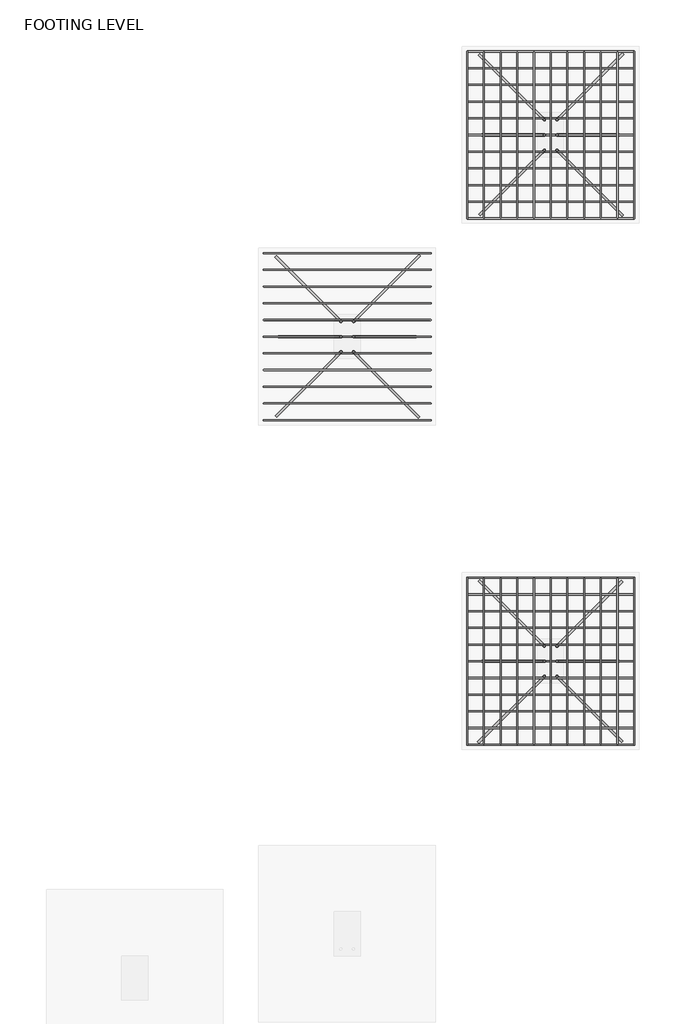
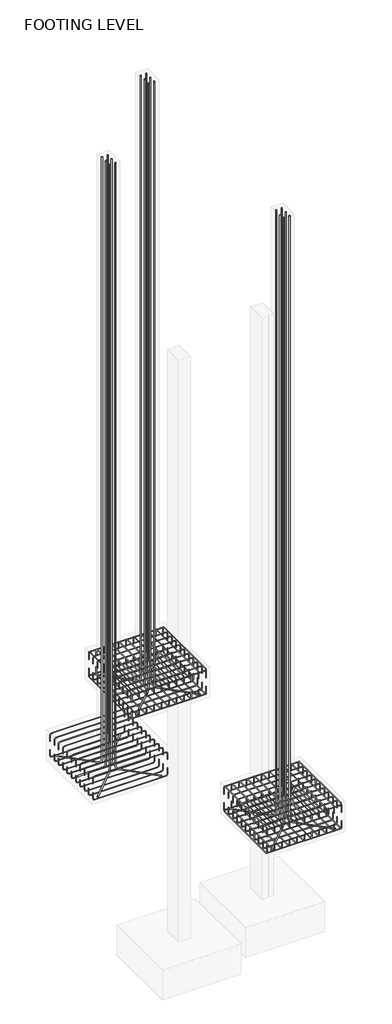
# One storey, part 10 of 10: 37 reinforcing bars.
"""IFC4 building model written with IfcOpenShell, lengths in millimetres."""

from ifc_helpers import new_model, si_unit, point, frame, origin, place, context, project, spatial, polyline, circle_curve, trimmed, segment, composite_curve, source, transform, mapped, element, save
from ifc_brep_helpers import swept_disk

model = new_model("IFC4")

# Units and contexts
model_context = context("Model", 3, world=origin())
ifc_project = project(units=[si_unit("LENGTHUNIT", "METRE", prefix="MILLI")], contexts=[model_context])

# Site, building, storey
site = spatial("IfcSite", under=ifc_project)
building = spatial("IfcBuilding", under=site)
storey = spatial("IfcBuildingStorey", under=building, Name="FOOTING LEVEL", Elevation=-1371.6)

# Reinforcing bars
placement = place(None, origin())
reinforcing_bar_shape = source(origin(), model_context, "Body", "SolidModel", [
    swept_disk(composite_curve([segment(polyline([(-5201.8793223, 10778.016297, -1770.864029), (-5201.8793223, 10778.016297, -1885.164029)]), True, "CONTINUOUS"), segment(trimmed(circle_curve(frame((-5168.5418223, 10778.016297, -1885.164029), z_axis=(0.0, -1.0, 0.0), x_axis=(-33.337500000000546, 0.0, 0.0)), 33.3375), [point((-5201.8793223, 10778.016297, -1885.164029))], [point((-5168.5418223, 10778.016297, -1918.501529))], True, "CARTESIAN"), True, "CONTINUOUS"), segment(polyline([(-5168.5418223, 10778.016297, -1918.501529), (-3796.9418223, 10778.016297, -1918.501529)]), True, "CONTINUOUS"), segment(trimmed(circle_curve(frame((-3796.9418223, 10778.016297, -1885.164029), z_axis=(0.0, -1.0, 0.0), x_axis=(0.0, 0.0, -33.337499999999864)), 33.3375), [point((-3796.9418223, 10778.016297, -1918.501529))], [point((-3763.6043223, 10778.016297, -1885.164029))], True, "CARTESIAN"), True, "CONTINUOUS"), segment(polyline([(-3763.6043223, 10778.016297, -1885.164029), (-3763.6043223, 10778.016297, -1770.864029)]), True, "CONTINUOUS")], self_intersect=False), 4.7625),
])
element("IfcReinforcingBar", 1, at=placement, inside=storey, context=model_context, shape_type="MappedRepresentation", body=[
    mapped(reinforcing_bar_shape, transform((0.0, 0.0, 0.0), x_axis=(1.0, 0.0, 0.0), y_axis=(0.0, 1.0, 0.0), z_axis=(0.0, 0.0, 1.0))),
    mapped(reinforcing_bar_shape, transform((0.0, 143.8275, 0.0), x_axis=(1.0, 0.0, 0.0), y_axis=(0.0, 1.0, 0.0), z_axis=(0.0, 0.0, 1.0))),
    mapped(reinforcing_bar_shape, transform((0.0, 287.655, 0.0), x_axis=(1.0, 0.0, 0.0), y_axis=(0.0, 1.0, 0.0), z_axis=(0.0, 0.0, 1.0))),
    mapped(reinforcing_bar_shape, transform((0.0, 431.4825, 0.0), x_axis=(1.0, 0.0, 0.0), y_axis=(0.0, 1.0, 0.0), z_axis=(0.0, 0.0, 1.0))),
    mapped(reinforcing_bar_shape, transform((0.0, 575.31, 0.0), x_axis=(1.0, 0.0, 0.0), y_axis=(0.0, 1.0, 0.0), z_axis=(0.0, 0.0, 1.0))),
    mapped(reinforcing_bar_shape, transform((0.0, 719.1375, 0.0), x_axis=(1.0, 0.0, 0.0), y_axis=(0.0, 1.0, 0.0), z_axis=(0.0, 0.0, 1.0))),
    mapped(reinforcing_bar_shape, transform((0.0, 862.965, 0.0), x_axis=(1.0, 0.0, 0.0), y_axis=(0.0, 1.0, 0.0), z_axis=(0.0, 0.0, 1.0))),
    mapped(reinforcing_bar_shape, transform((0.0, 1006.7925, 0.0), x_axis=(1.0, 0.0, 0.0), y_axis=(0.0, 1.0, 0.0), z_axis=(0.0, 0.0, 1.0))),
    mapped(reinforcing_bar_shape, transform((0.0, 1150.62, 0.0), x_axis=(1.0, 0.0, 0.0), y_axis=(0.0, 1.0, 0.0), z_axis=(0.0, 0.0, 1.0))),
    mapped(reinforcing_bar_shape, transform((0.0, 1294.4475, 0.0), x_axis=(1.0, 0.0, 0.0), y_axis=(0.0, 1.0, 0.0), z_axis=(0.0, 0.0, 1.0))),
    mapped(reinforcing_bar_shape, transform((0.0, 1438.275, 0.0), x_axis=(1.0, 0.0, 0.0), y_axis=(0.0, 1.0, 0.0), z_axis=(0.0, 0.0, 1.0))),
])
reinforcing_bar_2_shape = source(origin(), model_context, "Body", "SolidModel", [
    swept_disk(composite_curve([segment(polyline([(-5201.8793223, 12216.291297, -1586.5406765), (-5201.8793223, 12216.291297, -1472.2406765)]), True, "CONTINUOUS"), segment(trimmed(circle_curve(frame((-5168.5418223, 12216.291297, -1472.2406765), z_axis=(0.0, 1.0, 0.0), x_axis=(-33.337500000000546, 0.0, 0.0)), 33.3375), [point((-5201.8793223, 12216.291297, -1472.2406765))], [point((-5168.5418223, 12216.291297, -1438.9031765))], True, "CARTESIAN"), True, "CONTINUOUS"), segment(polyline([(-5168.5418223, 12216.291297, -1438.9031765), (-3796.9418223, 12216.291297, -1438.9031765)]), True, "CONTINUOUS"), segment(trimmed(circle_curve(frame((-3796.9418223, 12216.291297, -1472.2406765), z_axis=(0.0, 1.0, 0.0), x_axis=(0.0, 0.0, 33.33750000000009)), 33.3375), [point((-3796.9418223, 12216.291297, -1438.9031765))], [point((-3763.6043223, 12216.291297, -1472.2406765))], True, "CARTESIAN"), True, "CONTINUOUS"), segment(polyline([(-3763.6043223, 12216.291297, -1472.2406765), (-3763.6043223, 12216.291297, -1586.5406765)]), True, "CONTINUOUS")], self_intersect=False), 4.7625),
])
element("IfcReinforcingBar", 2, at=placement, inside=storey, context=model_context, shape_type="MappedRepresentation", body=[
    mapped(reinforcing_bar_2_shape, transform((0.0, 0.0, 0.0), x_axis=(1.0, 0.0, 0.0), y_axis=(0.0, 1.0, 0.0), z_axis=(0.0, 0.0, 1.0))),
    mapped(reinforcing_bar_2_shape, transform((0.0, -143.8275, 0.0), x_axis=(1.0, 0.0, 0.0), y_axis=(0.0, 1.0, 0.0), z_axis=(0.0, 0.0, 1.0))),
    mapped(reinforcing_bar_2_shape, transform((0.0, -287.655, 0.0), x_axis=(1.0, 0.0, 0.0), y_axis=(0.0, 1.0, 0.0), z_axis=(0.0, 0.0, 1.0))),
    mapped(reinforcing_bar_2_shape, transform((0.0, -431.4825, 0.0), x_axis=(1.0, 0.0, 0.0), y_axis=(0.0, 1.0, 0.0), z_axis=(0.0, 0.0, 1.0))),
    mapped(reinforcing_bar_2_shape, transform((0.0, -575.31, 0.0), x_axis=(1.0, 0.0, 0.0), y_axis=(0.0, 1.0, 0.0), z_axis=(0.0, 0.0, 1.0))),
    mapped(reinforcing_bar_2_shape, transform((0.0, -719.1375, 0.0), x_axis=(1.0, 0.0, 0.0), y_axis=(0.0, 1.0, 0.0), z_axis=(0.0, 0.0, 1.0))),
    mapped(reinforcing_bar_2_shape, transform((0.0, -862.965, 0.0), x_axis=(1.0, 0.0, 0.0), y_axis=(0.0, 1.0, 0.0), z_axis=(0.0, 0.0, 1.0))),
    mapped(reinforcing_bar_2_shape, transform((0.0, -1006.7925, 0.0), x_axis=(1.0, 0.0, 0.0), y_axis=(0.0, 1.0, 0.0), z_axis=(0.0, 0.0, 1.0))),
    mapped(reinforcing_bar_2_shape, transform((0.0, -1150.62, 0.0), x_axis=(1.0, 0.0, 0.0), y_axis=(0.0, 1.0, 0.0), z_axis=(0.0, 0.0, 1.0))),
    mapped(reinforcing_bar_2_shape, transform((0.0, -1294.4475, 0.0), x_axis=(1.0, 0.0, 0.0), y_axis=(0.0, 1.0, 0.0), z_axis=(0.0, 0.0, 1.0))),
    mapped(reinforcing_bar_2_shape, transform((0.0, -1438.275, 0.0), x_axis=(1.0, 0.0, 0.0), y_axis=(0.0, 1.0, 0.0), z_axis=(0.0, 0.0, 1.0))),
])
reinforcing_bar_3_shape = source(origin(), model_context, "Body", "SolidModel", [
    swept_disk(composite_curve([segment(polyline([(-2011.0043223, 13953.4953802, -1562.1), (-2011.0043223, 13953.4953802, -1447.8)]), True, "CONTINUOUS"), segment(trimmed(circle_curve(frame((-2011.0043223, 13920.1578802, -1447.8), z_axis=(1.0, 0.0, 0.0), x_axis=(0.0, 33.337499999999636, 0.0)), 33.3375), [point((-2011.0043223, 13953.4953802, -1447.8))], [point((-2011.0043223, 13920.1578802, -1414.4625))], True, "CARTESIAN"), True, "CONTINUOUS"), segment(polyline([(-2011.0043223, 13920.1578802, -1414.4625), (-2011.0043223, 12548.5578802, -1414.4625)]), True, "CONTINUOUS"), segment(trimmed(circle_curve(frame((-2011.0043223, 12548.5578802, -1447.8), z_axis=(1.0, 0.0, 0.0), x_axis=(0.0, 0.0, 33.337499999999864)), 33.3375), [point((-2011.0043223, 12548.5578802, -1414.4625))], [point((-2011.0043223, 12515.2203802, -1447.8))], True, "CARTESIAN"), True, "CONTINUOUS"), segment(polyline([(-2011.0043223, 12515.2203802, -1447.8), (-2011.0043223, 12515.2203802, -1562.1)]), True, "CONTINUOUS")], self_intersect=False), 4.7625),
])
element("IfcReinforcingBar", 3, at=placement, inside=storey, context=model_context, shape_type="MappedRepresentation", body=[
    mapped(reinforcing_bar_3_shape, transform((0.0, 0.0, 0.0), x_axis=(1.0, 0.0, 0.0), y_axis=(0.0, 1.0, 0.0), z_axis=(0.0, 0.0, 1.0))),
    mapped(reinforcing_bar_3_shape, transform((-143.8275, 0.0, 0.0), x_axis=(1.0, 0.0, 0.0), y_axis=(0.0, 1.0, 0.0), z_axis=(0.0, 0.0, 1.0))),
    mapped(reinforcing_bar_3_shape, transform((-287.655, 0.0, 0.0), x_axis=(1.0, 0.0, 0.0), y_axis=(0.0, 1.0, 0.0), z_axis=(0.0, 0.0, 1.0))),
    mapped(reinforcing_bar_3_shape, transform((-431.4825, 0.0, 0.0), x_axis=(1.0, 0.0, 0.0), y_axis=(0.0, 1.0, 0.0), z_axis=(0.0, 0.0, 1.0))),
    mapped(reinforcing_bar_3_shape, transform((-575.31, 0.0, 0.0), x_axis=(1.0, 0.0, 0.0), y_axis=(0.0, 1.0, 0.0), z_axis=(0.0, 0.0, 1.0))),
    mapped(reinforcing_bar_3_shape, transform((-719.1375, 0.0, 0.0), x_axis=(1.0, 0.0, 0.0), y_axis=(0.0, 1.0, 0.0), z_axis=(0.0, 0.0, 1.0))),
    mapped(reinforcing_bar_3_shape, transform((-862.965, 0.0, 0.0), x_axis=(1.0, 0.0, 0.0), y_axis=(0.0, 1.0, 0.0), z_axis=(0.0, 0.0, 1.0))),
    mapped(reinforcing_bar_3_shape, transform((-1006.7925, 0.0, 0.0), x_axis=(1.0, 0.0, 0.0), y_axis=(0.0, 1.0, 0.0), z_axis=(0.0, 0.0, 1.0))),
    mapped(reinforcing_bar_3_shape, transform((-1150.62, 0.0, 0.0), x_axis=(1.0, 0.0, 0.0), y_axis=(0.0, 1.0, 0.0), z_axis=(0.0, 0.0, 1.0))),
    mapped(reinforcing_bar_3_shape, transform((-1294.4475, 0.0, 0.0), x_axis=(1.0, 0.0, 0.0), y_axis=(0.0, 1.0, 0.0), z_axis=(0.0, 0.0, 1.0))),
    mapped(reinforcing_bar_3_shape, transform((-1438.275, 0.0, 0.0), x_axis=(1.0, 0.0, 0.0), y_axis=(0.0, 1.0, 0.0), z_axis=(0.0, 0.0, 1.0))),
])
reinforcing_bar_4_shape = source(origin(), model_context, "Body", "SolidModel", [
    swept_disk(composite_curve([segment(polyline([(-2011.0043223, 12515.2203802, -1790.7), (-2011.0043223, 12515.2203802, -1905.0)]), True, "CONTINUOUS"), segment(trimmed(circle_curve(frame((-2011.0043223, 12548.5578802, -1905.0), z_axis=(1.0, 0.0, 0.0), x_axis=(0.0, -33.337499999999636, 0.0)), 33.3375), [point((-2011.0043223, 12515.2203802, -1905.0))], [point((-2011.0043223, 12548.5578802, -1938.3375))], True, "CARTESIAN"), True, "CONTINUOUS"), segment(polyline([(-2011.0043223, 12548.5578802, -1938.3375), (-2011.0043223, 13920.1578802, -1938.3375)]), True, "CONTINUOUS"), segment(trimmed(circle_curve(frame((-2011.0043223, 13920.1578802, -1905.0), z_axis=(1.0, 0.0, 0.0), x_axis=(0.0, 0.0, -33.33750000000009)), 33.3375), [point((-2011.0043223, 13920.1578802, -1938.3375))], [point((-2011.0043223, 13953.4953802, -1905.0))], True, "CARTESIAN"), True, "CONTINUOUS"), segment(polyline([(-2011.0043223, 13953.4953802, -1905.0), (-2011.0043223, 13953.4953802, -1790.7)]), True, "CONTINUOUS")], self_intersect=False), 4.7625),
])
element("IfcReinforcingBar", 4, at=placement, inside=storey, context=model_context, shape_type="MappedRepresentation", body=[
    mapped(reinforcing_bar_4_shape, transform((0.0, 0.0, 0.0), x_axis=(1.0, 0.0, 0.0), y_axis=(0.0, 1.0, 0.0), z_axis=(0.0, 0.0, 1.0))),
    mapped(reinforcing_bar_4_shape, transform((-143.8275, 0.0, 0.0), x_axis=(1.0, 0.0, 0.0), y_axis=(0.0, 1.0, 0.0), z_axis=(0.0, 0.0, 1.0))),
    mapped(reinforcing_bar_4_shape, transform((-287.655, 0.0, 0.0), x_axis=(1.0, 0.0, 0.0), y_axis=(0.0, 1.0, 0.0), z_axis=(0.0, 0.0, 1.0))),
    mapped(reinforcing_bar_4_shape, transform((-431.4825, 0.0, 0.0), x_axis=(1.0, 0.0, 0.0), y_axis=(0.0, 1.0, 0.0), z_axis=(0.0, 0.0, 1.0))),
    mapped(reinforcing_bar_4_shape, transform((-575.31, 0.0, 0.0), x_axis=(1.0, 0.0, 0.0), y_axis=(0.0, 1.0, 0.0), z_axis=(0.0, 0.0, 1.0))),
    mapped(reinforcing_bar_4_shape, transform((-719.1375, 0.0, 0.0), x_axis=(1.0, 0.0, 0.0), y_axis=(0.0, 1.0, 0.0), z_axis=(0.0, 0.0, 1.0))),
    mapped(reinforcing_bar_4_shape, transform((-862.965, 0.0, 0.0), x_axis=(1.0, 0.0, 0.0), y_axis=(0.0, 1.0, 0.0), z_axis=(0.0, 0.0, 1.0))),
    mapped(reinforcing_bar_4_shape, transform((-1006.7925, 0.0, 0.0), x_axis=(1.0, 0.0, 0.0), y_axis=(0.0, 1.0, 0.0), z_axis=(0.0, 0.0, 1.0))),
    mapped(reinforcing_bar_4_shape, transform((-1150.62, 0.0, 0.0), x_axis=(1.0, 0.0, 0.0), y_axis=(0.0, 1.0, 0.0), z_axis=(0.0, 0.0, 1.0))),
    mapped(reinforcing_bar_4_shape, transform((-1294.4475, 0.0, 0.0), x_axis=(1.0, 0.0, 0.0), y_axis=(0.0, 1.0, 0.0), z_axis=(0.0, 0.0, 1.0))),
    mapped(reinforcing_bar_4_shape, transform((-1438.275, 0.0, 0.0), x_axis=(1.0, 0.0, 0.0), y_axis=(0.0, 1.0, 0.0), z_axis=(0.0, 0.0, 1.0))),
])
reinforcing_bar_5_shape = source(origin(), model_context, "Body", "SolidModel", [
    swept_disk(composite_curve([segment(polyline([(-3449.2793223, 12515.2203802, -1770.864029), (-3449.2793223, 12515.2203802, -1885.164029)]), True, "CONTINUOUS"), segment(trimmed(circle_curve(frame((-3415.9418223, 12515.2203802, -1885.164029), z_axis=(0.0, -1.0, 0.0), x_axis=(-33.33750000000009, 0.0, 0.0)), 33.3375), [point((-3449.2793223, 12515.2203802, -1885.164029))], [point((-3415.9418223, 12515.2203802, -1918.501529))], True, "CARTESIAN"), True, "CONTINUOUS"), segment(polyline([(-3415.9418223, 12515.2203802, -1918.501529), (-2044.3418223, 12515.2203802, -1918.501529)]), True, "CONTINUOUS"), segment(trimmed(circle_curve(frame((-2044.3418223, 12515.2203802, -1885.164029), z_axis=(0.0, -1.0, 0.0), x_axis=(0.0, 0.0, -33.337499999999864)), 33.3375), [point((-2044.3418223, 12515.2203802, -1918.501529))], [point((-2011.0043223, 12515.2203802, -1885.164029))], True, "CARTESIAN"), True, "CONTINUOUS"), segment(polyline([(-2011.0043223, 12515.2203802, -1885.164029), (-2011.0043223, 12515.2203802, -1770.864029)]), True, "CONTINUOUS")], self_intersect=False), 4.7625),
])
element("IfcReinforcingBar", 5, at=placement, inside=storey, context=model_context, shape_type="MappedRepresentation", body=[
    mapped(reinforcing_bar_5_shape, transform((0.0, 0.0, 0.0), x_axis=(1.0, 0.0, 0.0), y_axis=(0.0, 1.0, 0.0), z_axis=(0.0, 0.0, 1.0))),
    mapped(reinforcing_bar_5_shape, transform((0.0, 143.8275, 0.0), x_axis=(1.0, 0.0, 0.0), y_axis=(0.0, 1.0, 0.0), z_axis=(0.0, 0.0, 1.0))),
    mapped(reinforcing_bar_5_shape, transform((0.0, 287.655, 0.0), x_axis=(1.0, 0.0, 0.0), y_axis=(0.0, 1.0, 0.0), z_axis=(0.0, 0.0, 1.0))),
    mapped(reinforcing_bar_5_shape, transform((0.0, 431.4825, 0.0), x_axis=(1.0, 0.0, 0.0), y_axis=(0.0, 1.0, 0.0), z_axis=(0.0, 0.0, 1.0))),
    mapped(reinforcing_bar_5_shape, transform((0.0, 575.31, 0.0), x_axis=(1.0, 0.0, 0.0), y_axis=(0.0, 1.0, 0.0), z_axis=(0.0, 0.0, 1.0))),
    mapped(reinforcing_bar_5_shape, transform((0.0, 719.1375, 0.0), x_axis=(1.0, 0.0, 0.0), y_axis=(0.0, 1.0, 0.0), z_axis=(0.0, 0.0, 1.0))),
    mapped(reinforcing_bar_5_shape, transform((0.0, 862.965, 0.0), x_axis=(1.0, 0.0, 0.0), y_axis=(0.0, 1.0, 0.0), z_axis=(0.0, 0.0, 1.0))),
    mapped(reinforcing_bar_5_shape, transform((0.0, 1006.7925, 0.0), x_axis=(1.0, 0.0, 0.0), y_axis=(0.0, 1.0, 0.0), z_axis=(0.0, 0.0, 1.0))),
    mapped(reinforcing_bar_5_shape, transform((0.0, 1150.62, 0.0), x_axis=(1.0, 0.0, 0.0), y_axis=(0.0, 1.0, 0.0), z_axis=(0.0, 0.0, 1.0))),
    mapped(reinforcing_bar_5_shape, transform((0.0, 1294.4475, 0.0), x_axis=(1.0, 0.0, 0.0), y_axis=(0.0, 1.0, 0.0), z_axis=(0.0, 0.0, 1.0))),
    mapped(reinforcing_bar_5_shape, transform((0.0, 1438.275, 0.0), x_axis=(1.0, 0.0, 0.0), y_axis=(0.0, 1.0, 0.0), z_axis=(0.0, 0.0, 1.0))),
])
reinforcing_bar_6_shape = source(origin(), model_context, "Body", "SolidModel", [
    swept_disk(composite_curve([segment(polyline([(-3449.2793223, 13953.4953802, -1586.5406765), (-3449.2793223, 13953.4953802, -1472.2406765)]), True, "CONTINUOUS"), segment(trimmed(circle_curve(frame((-3415.9418223, 13953.4953802, -1472.2406765), z_axis=(0.0, 1.0, 0.0), x_axis=(-33.33750000000009, 0.0, 0.0)), 33.3375), [point((-3449.2793223, 13953.4953802, -1472.2406765))], [point((-3415.9418223, 13953.4953802, -1438.9031765))], True, "CARTESIAN"), True, "CONTINUOUS"), segment(polyline([(-3415.9418223, 13953.4953802, -1438.9031765), (-2044.3418223, 13953.4953802, -1438.9031765)]), True, "CONTINUOUS"), segment(trimmed(circle_curve(frame((-2044.3418223, 13953.4953802, -1472.2406765), z_axis=(0.0, 1.0, 0.0), x_axis=(0.0, 0.0, 33.33750000000009)), 33.3375), [point((-2044.3418223, 13953.4953802, -1438.9031765))], [point((-2011.0043223, 13953.4953802, -1472.2406765))], True, "CARTESIAN"), True, "CONTINUOUS"), segment(polyline([(-2011.0043223, 13953.4953802, -1472.2406765), (-2011.0043223, 13953.4953802, -1586.5406765)]), True, "CONTINUOUS")], self_intersect=False), 4.7625),
])
element("IfcReinforcingBar", 6, at=placement, inside=storey, context=model_context, shape_type="MappedRepresentation", body=[
    mapped(reinforcing_bar_6_shape, transform((0.0, 0.0, 0.0), x_axis=(1.0, 0.0, 0.0), y_axis=(0.0, 1.0, 0.0), z_axis=(0.0, 0.0, 1.0))),
    mapped(reinforcing_bar_6_shape, transform((0.0, -143.8275, 0.0), x_axis=(1.0, 0.0, 0.0), y_axis=(0.0, 1.0, 0.0), z_axis=(0.0, 0.0, 1.0))),
    mapped(reinforcing_bar_6_shape, transform((0.0, -287.655, 0.0), x_axis=(1.0, 0.0, 0.0), y_axis=(0.0, 1.0, 0.0), z_axis=(0.0, 0.0, 1.0))),
    mapped(reinforcing_bar_6_shape, transform((0.0, -431.4825, 0.0), x_axis=(1.0, 0.0, 0.0), y_axis=(0.0, 1.0, 0.0), z_axis=(0.0, 0.0, 1.0))),
    mapped(reinforcing_bar_6_shape, transform((0.0, -575.31, 0.0), x_axis=(1.0, 0.0, 0.0), y_axis=(0.0, 1.0, 0.0), z_axis=(0.0, 0.0, 1.0))),
    mapped(reinforcing_bar_6_shape, transform((0.0, -719.1375, 0.0), x_axis=(1.0, 0.0, 0.0), y_axis=(0.0, 1.0, 0.0), z_axis=(0.0, 0.0, 1.0))),
    mapped(reinforcing_bar_6_shape, transform((0.0, -862.965, 0.0), x_axis=(1.0, 0.0, 0.0), y_axis=(0.0, 1.0, 0.0), z_axis=(0.0, 0.0, 1.0))),
    mapped(reinforcing_bar_6_shape, transform((0.0, -1006.7925, 0.0), x_axis=(1.0, 0.0, 0.0), y_axis=(0.0, 1.0, 0.0), z_axis=(0.0, 0.0, 1.0))),
    mapped(reinforcing_bar_6_shape, transform((0.0, -1150.62, 0.0), x_axis=(1.0, 0.0, 0.0), y_axis=(0.0, 1.0, 0.0), z_axis=(0.0, 0.0, 1.0))),
    mapped(reinforcing_bar_6_shape, transform((0.0, -1294.4475, 0.0), x_axis=(1.0, 0.0, 0.0), y_axis=(0.0, 1.0, 0.0), z_axis=(0.0, 0.0, 1.0))),
    mapped(reinforcing_bar_6_shape, transform((0.0, -1438.275, 0.0), x_axis=(1.0, 0.0, 0.0), y_axis=(0.0, 1.0, 0.0), z_axis=(0.0, 0.0, 1.0))),
])
reinforcing_bar_7_shape = source(origin(), model_context, "Body", "SolidModel", [
    swept_disk(composite_curve([segment(polyline([(-3449.2793223, 7981.3203802, -1562.1), (-3449.2793223, 7981.3203802, -1447.8)]), True, "CONTINUOUS"), segment(trimmed(circle_curve(frame((-3449.2793223, 8014.6578802, -1447.8), z_axis=(-1.0, 0.0, 0.0), x_axis=(0.0, -33.337500000000546, 0.0)), 33.3375), [point((-3449.2793223, 7981.3203802, -1447.8))], [point((-3449.2793223, 8014.6578802, -1414.4625))], True, "CARTESIAN"), True, "CONTINUOUS"), segment(polyline([(-3449.2793223, 8014.6578802, -1414.4625), (-3449.2793223, 9386.2578802, -1414.4625)]), True, "CONTINUOUS"), segment(trimmed(circle_curve(frame((-3449.2793223, 9386.2578802, -1447.8), z_axis=(-1.0, 0.0, 0.0), x_axis=(0.0, 0.0, 33.337499999999864)), 33.3375), [point((-3449.2793223, 9386.2578802, -1414.4625))], [point((-3449.2793223, 9419.5953802, -1447.8))], True, "CARTESIAN"), True, "CONTINUOUS"), segment(polyline([(-3449.2793223, 9419.5953802, -1447.8), (-3449.2793223, 9419.5953802, -1562.1)]), True, "CONTINUOUS")], self_intersect=False), 4.7625),
])
element("IfcReinforcingBar", 7, at=placement, inside=storey, context=model_context, shape_type="MappedRepresentation", body=[
    mapped(reinforcing_bar_7_shape, transform((0.0, 0.0, 0.0), x_axis=(1.0, 0.0, 0.0), y_axis=(0.0, 1.0, 0.0), z_axis=(0.0, 0.0, 1.0))),
    mapped(reinforcing_bar_7_shape, transform((143.8275, 0.0, 0.0), x_axis=(1.0, 0.0, 0.0), y_axis=(0.0, 1.0, 0.0), z_axis=(0.0, 0.0, 1.0))),
    mapped(reinforcing_bar_7_shape, transform((287.655, 0.0, 0.0), x_axis=(1.0, 0.0, 0.0), y_axis=(0.0, 1.0, 0.0), z_axis=(0.0, 0.0, 1.0))),
    mapped(reinforcing_bar_7_shape, transform((431.4825, 0.0, 0.0), x_axis=(1.0, 0.0, 0.0), y_axis=(0.0, 1.0, 0.0), z_axis=(0.0, 0.0, 1.0))),
    mapped(reinforcing_bar_7_shape, transform((575.31, 0.0, 0.0), x_axis=(1.0, 0.0, 0.0), y_axis=(0.0, 1.0, 0.0), z_axis=(0.0, 0.0, 1.0))),
    mapped(reinforcing_bar_7_shape, transform((719.1375, 0.0, 0.0), x_axis=(1.0, 0.0, 0.0), y_axis=(0.0, 1.0, 0.0), z_axis=(0.0, 0.0, 1.0))),
    mapped(reinforcing_bar_7_shape, transform((862.965, 0.0, 0.0), x_axis=(1.0, 0.0, 0.0), y_axis=(0.0, 1.0, 0.0), z_axis=(0.0, 0.0, 1.0))),
    mapped(reinforcing_bar_7_shape, transform((1006.7925, 0.0, 0.0), x_axis=(1.0, 0.0, 0.0), y_axis=(0.0, 1.0, 0.0), z_axis=(0.0, 0.0, 1.0))),
    mapped(reinforcing_bar_7_shape, transform((1150.62, 0.0, 0.0), x_axis=(1.0, 0.0, 0.0), y_axis=(0.0, 1.0, 0.0), z_axis=(0.0, 0.0, 1.0))),
    mapped(reinforcing_bar_7_shape, transform((1294.4475, 0.0, 0.0), x_axis=(1.0, 0.0, 0.0), y_axis=(0.0, 1.0, 0.0), z_axis=(0.0, 0.0, 1.0))),
    mapped(reinforcing_bar_7_shape, transform((1438.275, 0.0, 0.0), x_axis=(1.0, 0.0, 0.0), y_axis=(0.0, 1.0, 0.0), z_axis=(0.0, 0.0, 1.0))),
])
reinforcing_bar_8_shape = source(origin(), model_context, "Body", "SolidModel", [
    swept_disk(composite_curve([segment(polyline([(-3449.2793223, 9419.5953802, -1790.7), (-3449.2793223, 9419.5953802, -1905.0)]), True, "CONTINUOUS"), segment(trimmed(circle_curve(frame((-3449.2793223, 9386.2578802, -1905.0), z_axis=(-1.0, 0.0, 0.0), x_axis=(0.0, 33.337499999999636, 0.0)), 33.3375), [point((-3449.2793223, 9419.5953802, -1905.0))], [point((-3449.2793223, 9386.2578802, -1938.3375))], True, "CARTESIAN"), True, "CONTINUOUS"), segment(polyline([(-3449.2793223, 9386.2578802, -1938.3375), (-3449.2793223, 8014.6578802, -1938.3375)]), True, "CONTINUOUS"), segment(trimmed(circle_curve(frame((-3449.2793223, 8014.6578802, -1905.0), z_axis=(-1.0, 0.0, 0.0), x_axis=(0.0, 0.0, -33.33750000000009)), 33.3375), [point((-3449.2793223, 8014.6578802, -1938.3375))], [point((-3449.2793223, 7981.3203802, -1905.0))], True, "CARTESIAN"), True, "CONTINUOUS"), segment(polyline([(-3449.2793223, 7981.3203802, -1905.0), (-3449.2793223, 7981.3203802, -1790.7)]), True, "CONTINUOUS")], self_intersect=False), 4.7625),
])
element("IfcReinforcingBar", 8, at=placement, inside=storey, context=model_context, shape_type="MappedRepresentation", body=[
    mapped(reinforcing_bar_8_shape, transform((0.0, 0.0, 0.0), x_axis=(1.0, 0.0, 0.0), y_axis=(0.0, 1.0, 0.0), z_axis=(0.0, 0.0, 1.0))),
    mapped(reinforcing_bar_8_shape, transform((143.8275, 0.0, 0.0), x_axis=(1.0, 0.0, 0.0), y_axis=(0.0, 1.0, 0.0), z_axis=(0.0, 0.0, 1.0))),
    mapped(reinforcing_bar_8_shape, transform((287.655, 0.0, 0.0), x_axis=(1.0, 0.0, 0.0), y_axis=(0.0, 1.0, 0.0), z_axis=(0.0, 0.0, 1.0))),
    mapped(reinforcing_bar_8_shape, transform((431.4825, 0.0, 0.0), x_axis=(1.0, 0.0, 0.0), y_axis=(0.0, 1.0, 0.0), z_axis=(0.0, 0.0, 1.0))),
    mapped(reinforcing_bar_8_shape, transform((575.31, 0.0, 0.0), x_axis=(1.0, 0.0, 0.0), y_axis=(0.0, 1.0, 0.0), z_axis=(0.0, 0.0, 1.0))),
    mapped(reinforcing_bar_8_shape, transform((719.1375, 0.0, 0.0), x_axis=(1.0, 0.0, 0.0), y_axis=(0.0, 1.0, 0.0), z_axis=(0.0, 0.0, 1.0))),
    mapped(reinforcing_bar_8_shape, transform((862.965, 0.0, 0.0), x_axis=(1.0, 0.0, 0.0), y_axis=(0.0, 1.0, 0.0), z_axis=(0.0, 0.0, 1.0))),
    mapped(reinforcing_bar_8_shape, transform((1006.7925, 0.0, 0.0), x_axis=(1.0, 0.0, 0.0), y_axis=(0.0, 1.0, 0.0), z_axis=(0.0, 0.0, 1.0))),
    mapped(reinforcing_bar_8_shape, transform((1150.62, 0.0, 0.0), x_axis=(1.0, 0.0, 0.0), y_axis=(0.0, 1.0, 0.0), z_axis=(0.0, 0.0, 1.0))),
    mapped(reinforcing_bar_8_shape, transform((1294.4475, 0.0, 0.0), x_axis=(1.0, 0.0, 0.0), y_axis=(0.0, 1.0, 0.0), z_axis=(0.0, 0.0, 1.0))),
    mapped(reinforcing_bar_8_shape, transform((1438.275, 0.0, 0.0), x_axis=(1.0, 0.0, 0.0), y_axis=(0.0, 1.0, 0.0), z_axis=(0.0, 0.0, 1.0))),
])
reinforcing_bar_9_shape = source(origin(), model_context, "Body", "SolidModel", [
    swept_disk(composite_curve([segment(polyline([(-2011.0043223, 9419.5953802, -1770.864029), (-2011.0043223, 9419.5953802, -1885.164029)]), True, "CONTINUOUS"), segment(trimmed(circle_curve(frame((-2044.3418223, 9419.5953802, -1885.164029), z_axis=(0.0, 1.0, 0.0), x_axis=(33.33750000000009, 0.0, 0.0)), 33.3375), [point((-2011.0043223, 9419.5953802, -1885.164029))], [point((-2044.3418223, 9419.5953802, -1918.501529))], True, "CARTESIAN"), True, "CONTINUOUS"), segment(polyline([(-2044.3418223, 9419.5953802, -1918.501529), (-3415.9418223, 9419.5953802, -1918.501529)]), True, "CONTINUOUS"), segment(trimmed(circle_curve(frame((-3415.9418223, 9419.5953802, -1885.164029), z_axis=(0.0, 1.0, 0.0), x_axis=(0.0, 0.0, -33.337499999999864)), 33.3375), [point((-3415.9418223, 9419.5953802, -1918.501529))], [point((-3449.2793223, 9419.5953802, -1885.164029))], True, "CARTESIAN"), True, "CONTINUOUS"), segment(polyline([(-3449.2793223, 9419.5953802, -1885.164029), (-3449.2793223, 9419.5953802, -1770.864029)]), True, "CONTINUOUS")], self_intersect=False), 4.7625),
])
element("IfcReinforcingBar", 9, at=placement, inside=storey, context=model_context, shape_type="MappedRepresentation", body=[
    mapped(reinforcing_bar_9_shape, transform((0.0, 0.0, 0.0), x_axis=(1.0, 0.0, 0.0), y_axis=(0.0, 1.0, 0.0), z_axis=(0.0, 0.0, 1.0))),
    mapped(reinforcing_bar_9_shape, transform((0.0, -143.8275, 0.0), x_axis=(1.0, 0.0, 0.0), y_axis=(0.0, 1.0, 0.0), z_axis=(0.0, 0.0, 1.0))),
    mapped(reinforcing_bar_9_shape, transform((0.0, -287.655, 0.0), x_axis=(1.0, 0.0, 0.0), y_axis=(0.0, 1.0, 0.0), z_axis=(0.0, 0.0, 1.0))),
    mapped(reinforcing_bar_9_shape, transform((0.0, -431.4825, 0.0), x_axis=(1.0, 0.0, 0.0), y_axis=(0.0, 1.0, 0.0), z_axis=(0.0, 0.0, 1.0))),
    mapped(reinforcing_bar_9_shape, transform((0.0, -575.31, 0.0), x_axis=(1.0, 0.0, 0.0), y_axis=(0.0, 1.0, 0.0), z_axis=(0.0, 0.0, 1.0))),
    mapped(reinforcing_bar_9_shape, transform((0.0, -719.1375, 0.0), x_axis=(1.0, 0.0, 0.0), y_axis=(0.0, 1.0, 0.0), z_axis=(0.0, 0.0, 1.0))),
    mapped(reinforcing_bar_9_shape, transform((0.0, -862.965, 0.0), x_axis=(1.0, 0.0, 0.0), y_axis=(0.0, 1.0, 0.0), z_axis=(0.0, 0.0, 1.0))),
    mapped(reinforcing_bar_9_shape, transform((0.0, -1006.7925, 0.0), x_axis=(1.0, 0.0, 0.0), y_axis=(0.0, 1.0, 0.0), z_axis=(0.0, 0.0, 1.0))),
    mapped(reinforcing_bar_9_shape, transform((0.0, -1150.62, 0.0), x_axis=(1.0, 0.0, 0.0), y_axis=(0.0, 1.0, 0.0), z_axis=(0.0, 0.0, 1.0))),
    mapped(reinforcing_bar_9_shape, transform((0.0, -1294.4475, 0.0), x_axis=(1.0, 0.0, 0.0), y_axis=(0.0, 1.0, 0.0), z_axis=(0.0, 0.0, 1.0))),
    mapped(reinforcing_bar_9_shape, transform((0.0, -1438.275, 0.0), x_axis=(1.0, 0.0, 0.0), y_axis=(0.0, 1.0, 0.0), z_axis=(0.0, 0.0, 1.0))),
])
reinforcing_bar_10_shape = source(origin(), model_context, "Body", "SolidModel", [
    swept_disk(composite_curve([segment(polyline([(-2011.0043223, 7981.3203802, -1586.5406765), (-2011.0043223, 7981.3203802, -1472.2406765)]), True, "CONTINUOUS"), segment(trimmed(circle_curve(frame((-2044.3418223, 7981.3203802, -1472.2406765), z_axis=(0.0, -1.0, 0.0), x_axis=(33.33750000000009, 0.0, 0.0)), 33.3375), [point((-2011.0043223, 7981.3203802, -1472.2406765))], [point((-2044.3418223, 7981.3203802, -1438.9031765))], True, "CARTESIAN"), True, "CONTINUOUS"), segment(polyline([(-2044.3418223, 7981.3203802, -1438.9031765), (-3415.9418223, 7981.3203802, -1438.9031765)]), True, "CONTINUOUS"), segment(trimmed(circle_curve(frame((-3415.9418223, 7981.3203802, -1472.2406765), z_axis=(0.0, -1.0, 0.0), x_axis=(0.0, 0.0, 33.33750000000009)), 33.3375), [point((-3415.9418223, 7981.3203802, -1438.9031765))], [point((-3449.2793223, 7981.3203802, -1472.2406765))], True, "CARTESIAN"), True, "CONTINUOUS"), segment(polyline([(-3449.2793223, 7981.3203802, -1472.2406765), (-3449.2793223, 7981.3203802, -1586.5406765)]), True, "CONTINUOUS")], self_intersect=False), 4.7625),
])
element("IfcReinforcingBar", 10, at=placement, inside=storey, context=model_context, shape_type="MappedRepresentation", body=[
    mapped(reinforcing_bar_10_shape, transform((0.0, 0.0, 0.0), x_axis=(1.0, 0.0, 0.0), y_axis=(0.0, 1.0, 0.0), z_axis=(0.0, 0.0, 1.0))),
    mapped(reinforcing_bar_10_shape, transform((0.0, 143.8275, 0.0), x_axis=(1.0, 0.0, 0.0), y_axis=(0.0, 1.0, 0.0), z_axis=(0.0, 0.0, 1.0))),
    mapped(reinforcing_bar_10_shape, transform((0.0, 287.655, 0.0), x_axis=(1.0, 0.0, 0.0), y_axis=(0.0, 1.0, 0.0), z_axis=(0.0, 0.0, 1.0))),
    mapped(reinforcing_bar_10_shape, transform((0.0, 431.4825, 0.0), x_axis=(1.0, 0.0, 0.0), y_axis=(0.0, 1.0, 0.0), z_axis=(0.0, 0.0, 1.0))),
    mapped(reinforcing_bar_10_shape, transform((0.0, 575.31, 0.0), x_axis=(1.0, 0.0, 0.0), y_axis=(0.0, 1.0, 0.0), z_axis=(0.0, 0.0, 1.0))),
    mapped(reinforcing_bar_10_shape, transform((0.0, 719.1375, 0.0), x_axis=(1.0, 0.0, 0.0), y_axis=(0.0, 1.0, 0.0), z_axis=(0.0, 0.0, 1.0))),
    mapped(reinforcing_bar_10_shape, transform((0.0, 862.965, 0.0), x_axis=(1.0, 0.0, 0.0), y_axis=(0.0, 1.0, 0.0), z_axis=(0.0, 0.0, 1.0))),
    mapped(reinforcing_bar_10_shape, transform((0.0, 1006.7925, 0.0), x_axis=(1.0, 0.0, 0.0), y_axis=(0.0, 1.0, 0.0), z_axis=(0.0, 0.0, 1.0))),
    mapped(reinforcing_bar_10_shape, transform((0.0, 1150.62, 0.0), x_axis=(1.0, 0.0, 0.0), y_axis=(0.0, 1.0, 0.0), z_axis=(0.0, 0.0, 1.0))),
    mapped(reinforcing_bar_10_shape, transform((0.0, 1294.4475, 0.0), x_axis=(1.0, 0.0, 0.0), y_axis=(0.0, 1.0, 0.0), z_axis=(0.0, 0.0, 1.0))),
    mapped(reinforcing_bar_10_shape, transform((0.0, 1438.275, 0.0), x_axis=(1.0, 0.0, 0.0), y_axis=(0.0, 1.0, 0.0), z_axis=(0.0, 0.0, 1.0))),
])
element("IfcReinforcingBar", 11, at=placement, inside=storey, context=model_context, shape_type="SolidModel", body=[
    swept_disk(composite_curve([segment(polyline([(-2675.7816302, 13364.9180723, -1333.5), (-2675.7816302, 13364.9180723, 10477.5)]), True, "CONTINUOUS")], self_intersect=False), 9.525),
])
element("IfcReinforcingBar", 12, at=placement, inside=storey, context=model_context, shape_type="SolidModel", body=[
    swept_disk(composite_curve([segment(polyline([(-2784.5020144, 13103.7976881, -1333.5), (-2784.5020144, 13103.7976881, 10477.5)]), True, "CONTINUOUS")], self_intersect=False), 9.525),
])
element("IfcReinforcingBar", 13, at=placement, inside=storey, context=model_context, shape_type="SolidModel", body=[
    swept_disk(composite_curve([segment(polyline([(-2675.7816302, 13103.7976881, -1333.5), (-2675.7816302, 13103.7976881, 10477.5)]), True, "CONTINUOUS")], self_intersect=False), 9.525),
])
element("IfcReinforcingBar", 14, at=placement, inside=storey, context=model_context, shape_type="SolidModel", body=[
    swept_disk(composite_curve([segment(polyline([(-3346.1777703, 13926.5938282, -1910.4342608), (-2831.648359, 13412.0644169, -1910.4342608)]), True, "CONTINUOUS"), segment(trimmed(circle_curve(frame((-2831.648359, 13412.0644169, -1843.7592608), z_axis=(-0.7071067811865736, -0.7071067811865216, 0.0), x_axis=(0.0, 0.0, -66.67499999999995)), 66.675), [point((-2831.648359, 13412.0644169, -1910.4342608))], [point((-2784.5020144, 13364.9180723, -1843.7592608))], True, "CARTESIAN"), True, "CONTINUOUS"), segment(polyline([(-2784.5020144, 13364.9180723, -1843.7592608), (-2784.5020144, 13364.9180723, 10477.5)]), True, "CONTINUOUS")], self_intersect=False), 9.525),
])
element("IfcReinforcingBar", 15, at=placement, inside=storey, context=model_context, shape_type="SolidModel", body=[
    swept_disk(composite_curve([segment(polyline([(-2106.0874965, 13934.612206, -1910.4342608), (-2628.6352856, 13412.0644169, -1910.4342608)]), True, "CONTINUOUS"), segment(trimmed(circle_curve(frame((-2628.6352856, 13412.0644169, -1843.7592608), z_axis=(-0.7071067811865712, 0.7071067811865238, 0.0), x_axis=(0.0, 0.0, -66.67499999999995)), 66.675), [point((-2628.6352856, 13412.0644169, -1910.4342608))], [point((-2675.7816302, 13364.9180723, -1843.7592608))], True, "CARTESIAN"), True, "CONTINUOUS"), segment(polyline([(-2675.7816302, 13364.9180723, -1843.7592608), (-2675.7816302, 13364.9180723, 10477.5)]), True, "CONTINUOUS")], self_intersect=False), 9.525),
])
element("IfcReinforcingBar", 16, at=placement, inside=storey, context=model_context, shape_type="SolidModel", body=[
    swept_disk(composite_curve([segment(polyline([(-3343.2211349, 12545.0785676, -1910.4342608), (-2831.648359, 13056.6513434, -1910.4342608)]), True, "CONTINUOUS"), segment(trimmed(circle_curve(frame((-2831.648359, 13056.6513434, -1843.7592608), z_axis=(0.707106781186576, -0.7071067811865192, 0.0), x_axis=(0.0, 0.0, -66.67499999999995)), 66.675), [point((-2831.648359, 13056.6513434, -1910.4342608))], [point((-2784.5020144, 13103.7976881, -1843.7592608))], True, "CARTESIAN"), True, "CONTINUOUS"), segment(polyline([(-2784.5020144, 13103.7976881, -1843.7592608), (-2784.5020144, 13103.7976881, 10477.5)]), True, "CONTINUOUS")], self_intersect=False), 9.525),
])
element("IfcReinforcingBar", 17, at=placement, inside=storey, context=model_context, shape_type="SolidModel", body=[
    swept_disk(composite_curve([segment(polyline([(-2111.6028099, 12539.6188678, -1910.4342608), (-2628.6352856, 13056.6513434, -1910.4342608)]), True, "CONTINUOUS"), segment(trimmed(circle_curve(frame((-2628.6352856, 13056.6513434, -1843.7592608), z_axis=(0.7071067811865689, 0.7071067811865261, 0.0), x_axis=(0.0, 0.0, -66.67499999999995)), 66.675), [point((-2628.6352856, 13056.6513434, -1910.4342608))], [point((-2675.7816302, 13103.7976881, -1843.7592608))], True, "CARTESIAN"), True, "CONTINUOUS"), segment(polyline([(-2675.7816302, 13103.7976881, -1843.7592608), (-2675.7816302, 13103.7976881, 10477.5)]), True, "CONTINUOUS")], self_intersect=False), 9.525),
])
element("IfcReinforcingBar", 18, at=placement, inside=storey, context=model_context, shape_type="SolidModel", body=[
    swept_disk(composite_curve([segment(polyline([(-3322.7318909, 13234.3578802, -1910.4342608), (-2851.1770144, 13234.3578802, -1910.4342608)]), True, "CONTINUOUS"), segment(trimmed(circle_curve(frame((-2851.1770144, 13234.3578802, -1843.7592608), z_axis=(0.0, -1.0, 0.0), x_axis=(0.0, 0.0, -66.67499999999995)), 66.675), [point((-2851.1770144, 13234.3578802, -1910.4342608))], [point((-2784.5020144, 13234.3578802, -1843.7592608))], True, "CARTESIAN"), True, "CONTINUOUS"), segment(polyline([(-2784.5020144, 13234.3578802, -1843.7592608), (-2784.5020144, 13234.3578802, 10477.5)]), True, "CONTINUOUS")], self_intersect=False), 9.525),
])
element("IfcReinforcingBar", 19, at=placement, inside=storey, context=model_context, shape_type="SolidModel", body=[
    swept_disk(composite_curve([segment(polyline([(-4428.3816302, 11627.7139891, -1333.5), (-4428.3816302, 11627.7139891, 10477.5)]), True, "CONTINUOUS")], self_intersect=False), 9.525),
])
element("IfcReinforcingBar", 20, at=placement, inside=storey, context=model_context, shape_type="SolidModel", body=[
    swept_disk(composite_curve([segment(polyline([(-4537.1020144, 11366.5936049, -1333.5), (-4537.1020144, 11366.5936049, 10477.5)]), True, "CONTINUOUS")], self_intersect=False), 9.525),
])
element("IfcReinforcingBar", 21, at=placement, inside=storey, context=model_context, shape_type="SolidModel", body=[
    swept_disk(composite_curve([segment(polyline([(-4428.3816302, 11366.5936049, -1333.5), (-4428.3816302, 11366.5936049, 10477.5)]), True, "CONTINUOUS")], self_intersect=False), 9.525),
])
element("IfcReinforcingBar", 22, at=placement, inside=storey, context=model_context, shape_type="SolidModel", body=[
    swept_disk(composite_curve([segment(polyline([(-5098.7777703, 12189.3897449, -1910.4342608), (-4584.2483591, 11674.8603337, -1910.4342608)]), True, "CONTINUOUS"), segment(trimmed(circle_curve(frame((-4584.2483591, 11674.8603337, -1843.7592608), z_axis=(-0.7071067811865736, -0.7071067811865216, 0.0), x_axis=(0.0, 0.0, -66.67499999999995)), 66.675), [point((-4584.2483591, 11674.8603337, -1910.4342608))], [point((-4537.1020144, 11627.7139891, -1843.7592608))], True, "CARTESIAN"), True, "CONTINUOUS"), segment(polyline([(-4537.1020144, 11627.7139891, -1843.7592608), (-4537.1020144, 11627.7139891, 10477.5)]), True, "CONTINUOUS")], self_intersect=False), 9.525),
])
element("IfcReinforcingBar", 23, at=placement, inside=storey, context=model_context, shape_type="SolidModel", body=[
    swept_disk(composite_curve([segment(polyline([(-3858.6874965, 12197.4081228, -1910.4342608), (-4381.2352856, 11674.8603337, -1910.4342608)]), True, "CONTINUOUS"), segment(trimmed(circle_curve(frame((-4381.2352856, 11674.8603337, -1843.7592608), z_axis=(-0.7071067811865712, 0.7071067811865238, 0.0), x_axis=(0.0, 0.0, -66.67499999999995)), 66.675), [point((-4381.2352856, 11674.8603337, -1910.4342608))], [point((-4428.3816302, 11627.7139891, -1843.7592608))], True, "CARTESIAN"), True, "CONTINUOUS"), segment(polyline([(-4428.3816302, 11627.7139891, -1843.7592608), (-4428.3816302, 11627.7139891, 10477.5)]), True, "CONTINUOUS")], self_intersect=False), 9.525),
])
element("IfcReinforcingBar", 24, at=placement, inside=storey, context=model_context, shape_type="SolidModel", body=[
    swept_disk(composite_curve([segment(polyline([(-5095.8211349, 10807.8744844, -1910.4342608), (-4584.2483591, 11319.4472602, -1910.4342608)]), True, "CONTINUOUS"), segment(trimmed(circle_curve(frame((-4584.2483591, 11319.4472602, -1843.7592608), z_axis=(0.707106781186576, -0.7071067811865192, 0.0), x_axis=(0.0, 0.0, -66.67499999999995)), 66.675), [point((-4584.2483591, 11319.4472602, -1910.4342608))], [point((-4537.1020144, 11366.5936049, -1843.7592608))], True, "CARTESIAN"), True, "CONTINUOUS"), segment(polyline([(-4537.1020144, 11366.5936049, -1843.7592608), (-4537.1020144, 11366.5936049, 10477.5)]), True, "CONTINUOUS")], self_intersect=False), 9.525),
])
element("IfcReinforcingBar", 25, at=placement, inside=storey, context=model_context, shape_type="SolidModel", body=[
    swept_disk(composite_curve([segment(polyline([(-3864.2028099, 10802.4147846, -1910.4342608), (-4381.2352856, 11319.4472602, -1910.4342608)]), True, "CONTINUOUS"), segment(trimmed(circle_curve(frame((-4381.2352856, 11319.4472602, -1843.7592608), z_axis=(0.7071067811865689, 0.7071067811865261, 0.0), x_axis=(0.0, 0.0, -66.67499999999995)), 66.675), [point((-4381.2352856, 11319.4472602, -1910.4342608))], [point((-4428.3816302, 11366.5936049, -1843.7592608))], True, "CARTESIAN"), True, "CONTINUOUS"), segment(polyline([(-4428.3816302, 11366.5936049, -1843.7592608), (-4428.3816302, 11366.5936049, 10477.5)]), True, "CONTINUOUS")], self_intersect=False), 9.525),
])
element("IfcReinforcingBar", 26, at=placement, inside=storey, context=model_context, shape_type="SolidModel", body=[
    swept_disk(composite_curve([segment(polyline([(-5075.3318909, 11497.153797, -1910.4342608), (-4603.7770144, 11497.153797, -1910.4342608)]), True, "CONTINUOUS"), segment(trimmed(circle_curve(frame((-4603.7770144, 11497.153797, -1843.7592608), z_axis=(0.0, -1.0, 0.0), x_axis=(0.0, 0.0, -66.67499999999995)), 66.675), [point((-4603.7770144, 11497.153797, -1910.4342608))], [point((-4537.1020144, 11497.153797, -1843.7592608))], True, "CARTESIAN"), True, "CONTINUOUS"), segment(polyline([(-4537.1020144, 11497.153797, -1843.7592608), (-4537.1020144, 11497.153797, 10477.5)]), True, "CONTINUOUS")], self_intersect=False), 9.525),
])
element("IfcReinforcingBar", 27, at=placement, inside=storey, context=model_context, shape_type="SolidModel", body=[
    swept_disk(composite_curve([segment(polyline([(-2784.5020144, 8569.8976881, -1333.5), (-2784.5020144, 8569.8976881, 10477.5)]), True, "CONTINUOUS")], self_intersect=False), 9.525),
])
element("IfcReinforcingBar", 28, at=placement, inside=storey, context=model_context, shape_type="SolidModel", body=[
    swept_disk(composite_curve([segment(polyline([(-2675.7816302, 8831.0180723, -1333.5), (-2675.7816302, 8831.0180723, 10477.5)]), True, "CONTINUOUS")], self_intersect=False), 9.525),
])
element("IfcReinforcingBar", 29, at=placement, inside=storey, context=model_context, shape_type="SolidModel", body=[
    swept_disk(composite_curve([segment(polyline([(-2784.5020144, 8831.0180723, -1333.5), (-2784.5020144, 8831.0180723, 10477.5)]), True, "CONTINUOUS")], self_intersect=False), 9.525),
])
element("IfcReinforcingBar", 30, at=placement, inside=storey, context=model_context, shape_type="SolidModel", body=[
    swept_disk(composite_curve([segment(polyline([(-2114.1058743, 8008.2219322, -1910.4342608), (-2628.6352856, 8522.7513434, -1910.4342608)]), True, "CONTINUOUS"), segment(trimmed(circle_curve(frame((-2628.6352856, 8522.7513434, -1843.7592608), z_axis=(0.7071067811865758, 0.7071067811865194, 0.0), x_axis=(0.0, 0.0, -66.67499999999995)), 66.675), [point((-2628.6352856, 8522.7513434, -1910.4342608))], [point((-2675.7816302, 8569.8976881, -1843.7592608))], True, "CARTESIAN"), True, "CONTINUOUS"), segment(polyline([(-2675.7816302, 8569.8976881, -1843.7592608), (-2675.7816302, 8569.8976881, 10477.5)]), True, "CONTINUOUS")], self_intersect=False), 9.525),
])
element("IfcReinforcingBar", 31, at=placement, inside=storey, context=model_context, shape_type="SolidModel", body=[
    swept_disk(composite_curve([segment(polyline([(-3354.1961481, 8000.2035544, -1910.4342608), (-2831.648359, 8522.7513434, -1910.4342608)]), True, "CONTINUOUS"), segment(trimmed(circle_curve(frame((-2831.648359, 8522.7513434, -1843.7592608), z_axis=(0.707106781186569, -0.707106781186526, 0.0), x_axis=(0.0, 0.0, -66.67499999999995)), 66.675), [point((-2831.648359, 8522.7513434, -1910.4342608))], [point((-2784.5020144, 8569.8976881, -1843.7592608))], True, "CARTESIAN"), True, "CONTINUOUS"), segment(polyline([(-2784.5020144, 8569.8976881, -1843.7592608), (-2784.5020144, 8569.8976881, 10477.5)]), True, "CONTINUOUS")], self_intersect=False), 9.525),
])
element("IfcReinforcingBar", 32, at=placement, inside=storey, context=model_context, shape_type="SolidModel", body=[
    swept_disk(composite_curve([segment(polyline([(-2117.0625098, 9389.7371927, -1910.4342608), (-2628.6352856, 8878.1644169, -1910.4342608)]), True, "CONTINUOUS"), segment(trimmed(circle_curve(frame((-2628.6352856, 8878.1644169, -1843.7592608), z_axis=(-0.7071067811865738, 0.7071067811865214, 0.0), x_axis=(0.0, 0.0, -66.67499999999995)), 66.675), [point((-2628.6352856, 8878.1644169, -1910.4342608))], [point((-2675.7816302, 8831.0180723, -1843.7592608))], True, "CARTESIAN"), True, "CONTINUOUS"), segment(polyline([(-2675.7816302, 8831.0180723, -1843.7592608), (-2675.7816302, 8831.0180723, 10477.5)]), True, "CONTINUOUS")], self_intersect=False), 9.525),
])
element("IfcReinforcingBar", 33, at=placement, inside=storey, context=model_context, shape_type="SolidModel", body=[
    swept_disk(composite_curve([segment(polyline([(-3348.6808347, 9395.1968926, -1910.4342608), (-2831.648359, 8878.1644169, -1910.4342608)]), True, "CONTINUOUS"), segment(trimmed(circle_curve(frame((-2831.648359, 8878.1644169, -1843.7592608), z_axis=(-0.7071067811865711, -0.7071067811865239, 0.0), x_axis=(0.0, 0.0, -66.67499999999995)), 66.675), [point((-2831.648359, 8878.1644169, -1910.4342608))], [point((-2784.5020144, 8831.0180723, -1843.7592608))], True, "CARTESIAN"), True, "CONTINUOUS"), segment(polyline([(-2784.5020144, 8831.0180723, -1843.7592608), (-2784.5020144, 8831.0180723, 10477.5)]), True, "CONTINUOUS")], self_intersect=False), 9.525),
])
element("IfcReinforcingBar", 34, at=placement, inside=storey, context=model_context, shape_type="SolidModel", body=[
    swept_disk(composite_curve([segment(polyline([(-2137.5517538, 8700.4578802, -1910.4342608), (-2609.1066302, 8700.4578802, -1910.4342608)]), True, "CONTINUOUS"), segment(trimmed(circle_curve(frame((-2609.1066302, 8700.4578802, -1843.7592608), z_axis=(0.0, 1.0, 0.0), x_axis=(0.0, 0.0, -66.67499999999995)), 66.675), [point((-2609.1066302, 8700.4578802, -1910.4342608))], [point((-2675.7816302, 8700.4578802, -1843.7592608))], True, "CARTESIAN"), True, "CONTINUOUS"), segment(polyline([(-2675.7816302, 8700.4578802, -1843.7592608), (-2675.7816302, 8700.4578802, 10477.5)]), True, "CONTINUOUS")], self_intersect=False), 9.525),
])
element("IfcReinforcingBar", 35, at=placement, inside=storey, context=model_context, shape_type="SolidModel", body=[
    swept_disk(composite_curve([segment(polyline([(-3322.7318909, 8700.4578802, -1916.7848067), (-2851.1770144, 8700.4578802, -1916.7848067)]), True, "CONTINUOUS"), segment(trimmed(circle_curve(frame((-2851.1770144, 8700.4578802, -1850.1098067), z_axis=(0.0, -1.0, 0.0), x_axis=(0.0, 0.0, -66.67499999999995)), 66.675), [point((-2851.1770144, 8700.4578802, -1916.7848067))], [point((-2784.5020144, 8700.4578802, -1850.1098067))], True, "CARTESIAN"), True, "CONTINUOUS"), segment(polyline([(-2784.5020144, 8700.4578802, -1850.1098067), (-2784.5020144, 8700.4578802, 10449.7223493)]), True, "CONTINUOUS")], self_intersect=False), 9.525),
])
element("IfcReinforcingBar", 36, at=placement, inside=storey, context=model_context, shape_type="SolidModel", body=[
    swept_disk(composite_curve([segment(polyline([(-3890.1517538, 11497.153797, -1910.4342608), (-4361.7066302, 11497.153797, -1910.4342608)]), True, "CONTINUOUS"), segment(trimmed(circle_curve(frame((-4361.7066302, 11497.153797, -1843.7592608), z_axis=(0.0, 1.0, 0.0), x_axis=(0.0, 0.0, -66.67499999999995)), 66.675), [point((-4361.7066302, 11497.153797, -1910.4342608))], [point((-4428.3816302, 11497.153797, -1843.7592608))], True, "CARTESIAN"), True, "CONTINUOUS"), segment(polyline([(-4428.3816302, 11497.153797, -1843.7592608), (-4428.3816302, 11497.153797, 10477.5)]), True, "CONTINUOUS")], self_intersect=False), 9.525),
])
element("IfcReinforcingBar", 37, at=placement, inside=storey, context=model_context, shape_type="SolidModel", body=[
    swept_disk(composite_curve([segment(polyline([(-2137.5517538, 13234.3578802, -1910.4342608), (-2609.1066302, 13234.3578802, -1910.4342608)]), True, "CONTINUOUS"), segment(trimmed(circle_curve(frame((-2609.1066302, 13234.3578802, -1843.7592608), z_axis=(0.0, 1.0, 0.0), x_axis=(0.0, 0.0, -66.67499999999995)), 66.675), [point((-2609.1066302, 13234.3578802, -1910.4342608))], [point((-2675.7816302, 13234.3578802, -1843.7592608))], True, "CARTESIAN"), True, "CONTINUOUS"), segment(polyline([(-2675.7816302, 13234.3578802, -1843.7592608), (-2675.7816302, 13234.3578802, 10477.5)]), True, "CONTINUOUS")], self_intersect=False), 9.525),
])

save(model, "model.ifc")

# Revit data of these elements
# Elements 1, 2, 3, 4, 5, 6, 7, 8, 9, 10, 11, 12, 13, 14, 15, 16, 17, 18, 19, 20, 21, 22, 23, 24, 25, 26, 27, 28, 29, 30, 31, 32, 33, 34, 35, 36, 37 (IfcReinforcingBar)
#   Phase Created = New Construction
